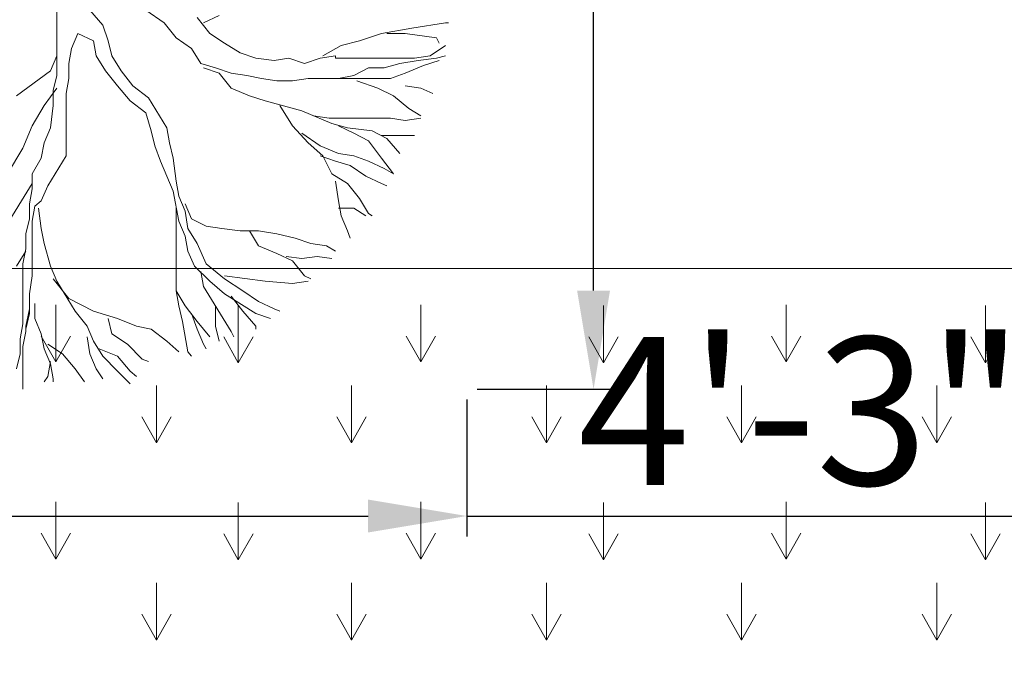
# Model space of a CAD drawing. Units: millimetres. Extents: x 595116 to 630915, y 909473 to 920225.
# Tile 50 of 134: x 629559 to 629619, y 919242 to 919281. Entities that reach past the tile are written whole.
import ezdxf

# ---------------------------------------------------------------- set-up
doc = ezdxf.new("R2010")
doc.units = ezdxf.units.MM
doc.layers.add('Dimension', color=3, linetype='Continuous', lineweight=18)
doc.layers.add('L-PLNT', color=85, linetype='Continuous', lineweight=13)
doc.styles.get("Standard").update_dxf_attribs({"font": 'arial.ttf'})
doc.dimstyles.new('ISO-25', dxfattribs={"dimtxt": 9, "dimasz": 6, "dimexe": 1.25, "dimexo": 0.625, "dimtad": 1, "dimlunit": 4, "dimtxsty": 'Standard', "dimcen": 2.5, "dimadec": 0, "dimazin": 0, "dimtfac": 1, "dimtmove": 0, "dimatfit": 3, "dimfxl": 1, "dimarcsym": 0})

# ---------------------------------------------------------------- blocks, each defined once
blk = doc.blocks.new('A$C143125F4')
for p, q in [((2.5383, 1.8726), (2.5383, 2.3206)), ((2.7353, 2.2623), (2.8119, 2.1727)), ((3.1784, 2.1862), (3.069, 2.2623)), ((3.2495, 2.0966), (3.1784, 2.1862)), ((3.4519, 2.1235), (3.3753, 2.2175)), ((3.4136, 2.1862), (3.5066, 2.231)), ((4.6554, 2.1548), (4.8578, 2.1862)), ((4.8578, 2.1862), (4.8742, 2.1862)), ((2.6641, 2.1235), (2.6259, 2.0339)), ((2.7571, 2.0787), (2.6641, 2.1235)), ((2.8119, 2.1727), (2.8447, 2.0787)), ((3.5394, 2.0652), (3.4519, 2.1235)), ((4.3436, 2.0787), (4.4749, 2.1235)), ((4.4749, 2.1235), (4.6554, 2.1548)), ((4.5077, 2.1235), (4.6171, 2.1235)), ((4.6171, 2.1235), (4.8031, 2.0966)), ((2.7736, 1.9891), (2.7571, 2.0787)), ((2.8447, 2.0787), (2.8666, 1.9891)), ((3.3425, 2.0339), (3.2495, 2.0966)), ((3.6324, 2.007), (3.5394, 2.0652)), ((4.2342, 2.0518), (4.3436, 2.0787)), ((4.8031, 2.0966), (4.8195, 2.0652)), ((2.6259, 2.0339), (2.6094, 1.9443)), ((3.3972, 1.9443), (3.3425, 2.0339)), ((3.7254, 1.9756), (3.6324, 2.007)), ((4.1248, 1.9891), (4.2342, 2.0518)), ((4.8578, 2.0518), (4.7648, 1.9891)), ((2.5383, 1.9891), (2.5, 1.8995)), ((2.6094, 1.9443), (2.6094, 1.8547)), ((2.8283, 1.8995), (2.7736, 1.9891)), ((2.8666, 1.9891), (2.9213, 1.8995)), ((3.4847, 1.9174), (3.3972, 1.9443)), ((3.8348, 1.9622), (3.7254, 1.9756)), ((3.9224, 1.9756), (3.8348, 1.9622)), ((4.0154, 1.9443), (3.9224, 1.9756)), ((4.1084, 1.9756), (4.0154, 1.9443)), ((4.2014, 1.9891), (4.1084, 1.9756)), ((4.2014, 1.9756), (4.2014, 1.9891)), ((4.6718, 1.9756), (4.2014, 1.9756)), ((4.4913, 1.9174), (4.5843, 1.9443)), ((4.5843, 1.9443), (4.6937, 1.9622)), ((4.7648, 1.9891), (4.6718, 1.9756)), ((4.6937, 1.9622), (4.8031, 1.9756)), ((4.8195, 1.9622), (4.7265, 1.9308)), ((4.8031, 1.9756), (4.8578, 1.9891)), ((2.5, 1.8995), (2.2976, 1.7516)), ((2.8994, 1.8099), (2.8283, 1.8995)), ((2.9213, 1.8995), (2.9924, 1.8099)), ((3.4136, 1.9174), (3.5066, 1.886)), ((3.5777, 1.886), (3.4847, 1.9174)), ((3.5066, 1.886), (3.5777, 1.7964)), ((3.6707, 1.8726), (3.5777, 1.886)), ((4.3108, 1.8726), (4.3983, 1.9174)), ((4.3983, 1.9174), (4.4913, 1.9174)), ((4.6171, 1.886), (4.5296, 1.8547)), ((4.7265, 1.9308), (4.6171, 1.886)), ((2.5164, 1.783), (2.5383, 1.8726)), ((2.6094, 1.8547), (2.593, 1.7651)), ((3.7583, 1.8547), (3.6707, 1.8726)), ((3.8512, 1.8412), (3.7583, 1.8547)), ((3.9442, 1.8412), (3.8512, 1.8412)), ((4.0372, 1.8547), (3.9442, 1.8412)), ((4.1248, 1.8547), (4.0372, 1.8547)), ((4.5296, 1.8547), (4.1248, 1.8547)), ((4.2178, 1.8547), (4.3108, 1.8726)), ((4.3272, 1.8412), (4.453, 1.7964)), ((2.5383, 1.7964), (2.4617, 1.6934)), ((2.5164, 1.6934), (2.5164, 1.783)), ((2.593, 1.7651), (2.593, 1.3932)), ((2.976, 1.7203), (2.8994, 1.8099)), ((2.9924, 1.8099), (3.0854, 1.7382)), ((3.5777, 1.7964), (3.6871, 1.7516)), ((4.453, 1.7964), (4.546, 1.7516)), ((4.6171, 1.8099), (4.7101, 1.7964)), ((4.7101, 1.7964), (4.7812, 1.7651)), ((3.069, 1.6486), (2.976, 1.7203)), ((3.0854, 1.7382), (3.1948, 1.559)), ((3.6871, 1.7516), (3.7801, 1.7203)), ((3.7801, 1.7203), (3.999, 1.662)), ((4.546, 1.7516), (4.639, 1.6755)), ((2.4617, 1.6934), (2.3906, 1.5724)), ((2.5, 1.559), (2.5164, 1.6934)), ((3.1018, 1.5411), (3.069, 1.6486)), ((3.8677, 1.6934), (3.9442, 1.5724)), ((3.999, 1.662), (4.1795, 1.5859)), ((4.639, 1.6755), (4.7101, 1.6307)), ((4.0701, 1.6307), (4.1631, 1.6172)), ((4.1631, 1.6172), (4.5296, 1.6172)), ((4.5296, 1.6172), (4.6171, 1.6038)), ((4.6171, 1.6038), (4.7101, 1.6172)), ((2.3906, 1.5724), (2.3359, 1.438)), ((2.4617, 1.4694), (2.5, 1.559)), ((3.1237, 1.4515), (3.1018, 1.5411)), ((3.1948, 1.559), (3.2112, 1.4694)), ((3.9442, 1.5724), (4.0372, 1.4694)), ((3.999, 1.5276), (4.1084, 1.4515)), ((4.1795, 1.5859), (4.2725, 1.559)), ((4.2178, 1.5724), (4.3108, 1.5276)), ((4.2725, 1.559), (4.4202, 1.5411)), ((4.3108, 1.5276), (4.3983, 1.4828)), ((4.4202, 1.5411), (4.5077, 1.4963)), ((2.4453, 1.3798), (2.4617, 1.4694)), ((3.2112, 1.4694), (3.2331, 1.3798)), ((4.0372, 1.4694), (4.1248, 1.3932)), ((4.3983, 1.4828), (4.4749, 1.3798)), ((4.4749, 1.5142), (4.6718, 1.5142)), ((4.5077, 1.4963), (4.5843, 1.4067)), ((2.3359, 1.438), (2.2429, 1.2857)), ((3.1565, 1.3619), (3.1237, 1.4515)), ((4.1084, 1.4515), (4.2178, 1.4067)), ((2.3906, 1.2857), (2.4453, 1.3798)), ((2.593, 1.3932), (2.4836, 1.214)), ((3.2331, 1.1827), (3.1565, 1.3619)), ((3.2331, 1.3798), (3.2495, 1.2409)), ((4.1084, 1.3932), (4.2014, 1.3619)), ((4.1248, 1.3932), (4.1795, 1.2857)), ((4.2014, 1.3619), (4.2889, 1.335)), ((4.2178, 1.4067), (4.3108, 1.3932)), ((4.3108, 1.3932), (4.3983, 1.3619)), ((4.3983, 1.3619), (4.4913, 1.3171)), ((4.4749, 1.3798), (4.546, 1.2857)), ((4.2889, 1.335), (4.3819, 1.2723)), ((4.4913, 1.3171), (4.546, 1.2857)), ((2.3906, 1.1961), (2.3906, 1.2857)), ((3.2495, 1.2409), (3.2659, 1.1513)), ((4.1795, 1.2857), (4.2725, 1.2275)), ((4.2014, 1.2409), (4.2178, 1.1244)), ((4.3819, 1.2723), (4.4749, 1.2275)), ((2.3906, 1.2275), (2.2265, 0.9587)), ((2.3742, 1.1065), (2.3906, 1.1961)), ((2.4836, 1.214), (2.4453, 1.1244)), ((3.2659, 1.0035), (3.2331, 1.1827)), ((4.2725, 1.2275), (4.3436, 1.1379)), ((4.4749, 1.2275), (4.5077, 1.214)), ((2.4453, 1.1244), (2.407, 1.0931)), ((3.2659, 1.1513), (3.3042, 1.0617)), ((4.2178, 1.1244), (4.2342, 1.0348)), ((4.3436, 1.1379), (4.3983, 1.0483)), ((2.3742, 1.0169), (2.3742, 1.1065)), ((2.407, 1.0931), (2.3906, 1.0035)), ((2.4289, 1.0796), (2.4453, 0.9587)), ((3.2495, 1.0796), (3.2495, 0.5869)), ((3.3042, 1.1065), (3.3425, 1.0169)), ((3.3042, 1.0617), (3.3206, 0.9587)), ((4.2178, 1.0796), (4.3108, 1.0796)), ((4.3108, 1.0796), (4.3819, 1.0348)), ((2.3523, 0.9273), (2.3742, 1.0169)), ((2.3906, 1.0035), (2.3906, 0.6765)), ((3.3042, 0.9139), (3.2659, 1.0035)), ((3.3425, 1.0169), (3.43, 0.9721)), ((4.2342, 1.0348), (4.2725, 0.9452)), ((4.3983, 1.0483), (4.4202, 1.0348)), ((2.4453, 0.9587), (2.4617, 0.8691)), ((3.3206, 0.9587), (3.3753, 0.8691)), ((3.43, 0.9721), (3.523, 0.9587)), ((3.523, 0.9587), (3.6324, 0.9452)), ((3.6324, 0.9452), (3.7418, 0.9452)), ((3.6871, 0.9452), (3.7418, 0.8557)), ((3.7418, 0.9452), (3.8512, 0.9273)), ((4.2725, 0.9452), (4.2889, 0.9005)), ((2.3523, 0.8377), (2.3523, 0.9273)), ((3.3206, 0.8243), (3.3042, 0.9139)), ((3.8512, 0.9273), (3.9607, 0.9005)), ((3.9607, 0.9005), (4.0537, 0.8691)), ((2.3523, 0.8243), (2.2976, 0.7347)), ((2.3359, 0.7481), (2.3523, 0.8377)), ((2.4617, 0.8691), (2.5, 0.7347)), ((3.3589, 0.7347), (3.3206, 0.8243)), ((3.3753, 0.8691), (3.43, 0.7481)), ((3.7418, 0.8557), (3.8512, 0.8109)), ((4.0537, 0.8691), (4.1467, 0.8557)), ((4.1467, 0.8557), (4.2014, 0.8243)), ((3.8512, 0.8109), (3.9442, 0.7661)), ((3.906, 0.7929), (3.999, 0.7795)), ((3.9442, 0.7661), (4.0154, 0.6765)), ((3.999, 0.7795), (4.092, 0.7929)), ((4.092, 0.7929), (4.1795, 0.7795)), ((2.3359, 0.3897), (2.3359, 0.7481)), ((2.5, 0.7347), (2.5383, 0.6451)), ((3.4519, 0.6451), (3.3589, 0.7347)), ((3.43, 0.7481), (3.5394, 0.6585)), ((2.3906, 0.6765), (2.3742, 0.5689)), ((2.5164, 0.6585), (2.6094, 0.5421)), ((3.3972, 0.7033), (3.4136, 0.6137)), ((3.5394, 0.6765), (3.7801, 0.6451)), ((3.5394, 0.6585), (3.6488, 0.5869)), ((4.0154, 0.6765), (4.0537, 0.6585)), ((2.5383, 0.6451), (2.6477, 0.4659)), ((3.4136, 0.6137), (3.5777, 0.3449)), ((3.5394, 0.5689), (3.4519, 0.6451)), ((3.7801, 0.6451), (3.9442, 0.6317)), ((3.9442, 0.6317), (4.0372, 0.6451)), ((2.3742, 0.5689), (2.3742, 0.4525)), ((2.6094, 0.5421), (2.7571, 0.4659)), ((3.2495, 0.5869), (3.3042, 0.4973)), ((3.2495, 0.5869), (3.2659, 0.4973)), ((3.7254, 0.4525), (3.5394, 0.5689)), ((3.5777, 0.5555), (3.6488, 0.4659)), ((3.6488, 0.5869), (3.7418, 0.5241)), ((2.3523, 0.3584), (2.3742, 0.4793)), ((2.3742, 0.4793), (2.3523, 0.3763)), ((2.407, 0.5107), (2.407, 0.4211)), ((3.2659, 0.4973), (3.2878, 0.4032)), ((3.3042, 0.4973), (3.3753, 0.4032)), ((3.4847, 0.4973), (3.4847, 0.3763)), ((3.7418, 0.5241), (3.8348, 0.4793)), ((3.8348, 0.4793), (3.8677, 0.4659)), ((2.3742, 0.4525), (2.3523, 0.3584)), ((2.407, 0.4211), (2.4453, 0.3315)), ((2.6477, 0.4659), (2.7189, 0.3763)), ((2.7571, 0.4659), (2.8994, 0.4211)), ((2.8447, 0.4211), (2.8666, 0.3315)), ((2.8994, 0.4211), (3.0143, 0.3763)), ((3.3425, 0.4525), (3.3753, 0.3584)), ((3.6488, 0.4659), (3.7254, 0.3763)), ((3.813, 0.4211), (3.7254, 0.4525)), ((2.3195, 0.3002), (2.3359, 0.3897)), ((2.3523, 0.3763), (2.3523, 0.3449)), ((2.7189, 0.3763), (2.7571, 0.2867)), ((3.0143, 0.3763), (3.1018, 0.3584)), ((3.1018, 0.3584), (3.1948, 0.2867)), ((3.2878, 0.4032), (3.3206, 0.224)), ((3.3753, 0.4032), (3.4519, 0.3136)), ((3.3753, 0.3584), (3.4136, 0.2688)), ((3.4847, 0.3763), (3.5066, 0.2867)), ((3.7254, 0.3763), (3.7254, 0.3584)), ((2.3195, 0.2106), (2.3195, 0.3002)), ((2.3523, 0.3449), (2.3359, 0.2554)), ((2.4453, 0.3315), (2.4617, 0.2419)), ((2.7189, 0.3136), (2.7353, 0.2106)), ((2.8666, 0.3315), (2.9596, 0.2688)), ((3.5777, 0.3449), (3.5941, 0.3136)), ((2.3359, 0.2554), (2.3359, 0)), ((2.4617, 0.2419), (2.5, 0.1523)), ((2.4836, 0.2688), (2.5711, 0.2106)), ((2.7571, 0.2867), (2.8119, 0.1971)), ((2.79, 0.2419), (2.8994, 0.1971)), ((2.9596, 0.2688), (3.0471, 0.1792)), ((3.1948, 0.2867), (3.2659, 0.224)), ((3.4136, 0.2688), (3.43, 0.2419)), ((2.2976, 0.121), (2.3195, 0.2106)), ((2.5711, 0.2106), (2.6477, 0.121)), ((2.7353, 0.2106), (2.7736, 0.121)), ((2.8119, 0.1971), (2.8994, 0.1075)), ((2.8994, 0.1971), (2.976, 0.1075)), ((3.0471, 0.1792), (3.0854, 0.1658)), ((3.3206, 0.224), (3.3425, 0.1971)), ((2.5, 0.1658), (2.4836, 0.0762)), ((2.5, 0.1523), (2.5164, 0.0627)), ((2.6477, 0.121), (2.7024, 0.0448)), ((2.7736, 0.121), (2.8119, 0.0627)), ((2.4836, 0.0762), (2.4617, 0.0448)), ((2.5164, 0.0627), (2.5164, 0.0448)), ((2.8994, 0.1075), (2.976, 0.0314)), ((2.976, 0.1075), (3.0143, 0.0762))]:
    blk.add_line(p, q)
blk = doc.blocks.new('LAWN-GRASS-TUFT')
blk.add_line((0.892, 3.485), (0.892, 0))
blk.add_lwpolyline([(0, 1.577), (0.892, 0), (1.785, 1.577)])
blk = doc.blocks.new('*D210')
at = {"layer": 'Defpoints', "color": 0, "transparency": 16777216}
for p in [(629586.227, 919310.123), (629593.946, 919310.123), (629586.227, 919258.662)]:
    blk.add_point(p, dxfattribs=at)
at = {"layer": 'Dimension', "color": 0, "lineweight": -2, "transparency": 16777216}
for p, q in [((629593.946, 919310.123), (629593.946, 919449.69)), ((629586.852, 919310.123), (629595.196, 919310.123)), ((629593.946, 919264.662), (629593.946, 919304.123)), ((629586.852, 919258.662), (629595.196, 919258.662))]:
    blk.add_line(p, q, dxfattribs=at)
at = {"layer": 'Dimension', "color": 0, "transparency": 16777216}
for points in [[(629592.946, 919304.123), (629594.946, 919304.123), (629593.946, 919310.123)], [(629592.946, 919264.662), (629594.946, 919264.662), (629593.946, 919258.662)]]:
    blk.add_solid(points, dxfattribs=at)
at = {"layer": 'Dimension', "color": 0, "transparency": 16777216, "insert": (629588.662, 919382.907), "char_height": 9, "attachment_point": 5, "rotation": 90}
blk.add_mtext('CANOPY 4\'-3 1/2" TYP.', dxfattribs=at)
blk = doc.blocks.new('*D211')
at = {"layer": 'Defpoints', "color": 0, "transparency": 16777216}
for p in [(629535.386, 919258.662), (629586.227, 919258.662), (629586.227, 919250.943)]:
    blk.add_point(p, dxfattribs=at)
at = {"layer": 'Dimension', "color": 0, "lineweight": -2, "transparency": 16777216}
for p, q in [((629535.386, 919258.037), (629535.386, 919249.693)), ((629586.227, 919258.037), (629586.227, 919249.693)), ((629541.386, 919250.943), (629580.227, 919250.943)), ((629586.227, 919250.943), (629648.699, 919250.943))]:
    blk.add_line(p, q, dxfattribs=at)
at = {"layer": 'Dimension', "color": 0, "transparency": 16777216}
for points in [[(629541.386, 919251.943), (629541.386, 919249.943), (629535.386, 919250.943)], [(629580.227, 919251.943), (629580.227, 919249.943), (629586.227, 919250.943)]]:
    blk.add_solid(points, dxfattribs=at)
at = {"layer": 'Dimension', "color": 0, "transparency": 16777216, "insert": (629620.463, 919256.167), "char_height": 9, "attachment_point": 5}
blk.add_mtext('4\'-3" TYP.', dxfattribs=at)
blk = doc.blocks.new('*D216')
at = {"layer": 'Defpoints', "color": 0, "transparency": 16777216}
for p in [(629505.041, 919411.828), (629743.541, 919411.928), (629743.541, 918832.378)]:
    blk.add_point(p, dxfattribs=at)
at = {"layer": 'Dimension', "color": 0, "lineweight": -2, "transparency": 16777216}
for p, q in [((629505.041, 919411.203), (629505.041, 918831.128)), ((629743.541, 919411.303), (629743.541, 918831.128)), ((629511.041, 918832.378), (629737.541, 918832.378))]:
    blk.add_line(p, q, dxfattribs=at)
at = {"layer": 'Dimension', "color": 0, "transparency": 16777216}
for points in [[(629511.041, 918833.378), (629511.041, 918831.378), (629505.041, 918832.378)], [(629737.541, 918833.378), (629737.541, 918831.378), (629743.541, 918832.378)]]:
    blk.add_solid(points, dxfattribs=at)
at = {"layer": 'Dimension', "color": 0, "transparency": 16777216, "insert": (629624.291, 918837.656), "char_height": 9, "attachment_point": 5}
blk.add_mtext('19\'-10 1/2"', dxfattribs=at)

msp = doc.modelspace()

# ---------------------------------------------------------------- linework, layer by layer
at = {"layer": 'L-PLNT'}
msp.add_line((629800.951, 919266.009), (629535.274, 919266.009), dxfattribs=at)

# ---------------------------------------------------------------- block references
at = {"layer": 'L-PLNT', "xscale": 10.20167662382051, "yscale": 10.20167662382051, "zscale": 10.20167662382051}
msp.add_blockref('A$C143125F4', (629535.386, 919258.662), dxfattribs=at)
at = {"layer": 'L-PLNT'}
for p in [(629560.321, 919260.324), (629571.434, 919260.275), (629582.548, 919260.324), (629593.662, 919260.275), (629604.776, 919260.324), (629616.912, 919260.275), (629566.446, 919255.397), (629578.319, 919255.397), (629590.192, 919255.397), (629602.065, 919255.397), (629613.938, 919255.397), (629560.321, 919248.322), (629571.434, 919248.272), (629582.548, 919248.322), (629593.662, 919248.272), (629604.776, 919248.322), (629616.912, 919248.272), (629566.446, 919243.395), (629578.319, 919243.395), (629590.192, 919243.395), (629602.065, 919243.395), (629613.938, 919243.395)]:
    msp.add_blockref('LAWN-GRASS-TUFT', p, dxfattribs=at)

# ---------------------------------------------------------------- dimensions: what is measured, and where the dimension line sits
at = {"layer": 'Dimension'}
dim = msp.add_linear_dim(base=(629593.946, 919310.123), p1=(629586.227, 919258.662), p2=(629586.227, 919310.123), angle=90, text='CANOPY <> TYP.', dimstyle='ISO-25', override={"dimdec": 1, "dimlfac": 1, "dimrnd": 0, "dimzin": 1, "dimdsep": 46, "dimlunit": 4, "dimfrac": 2}, dxfattribs=at)
dim.commit()
dim.dimension.update_dxf_attribs({"geometry": '*D210', "text_midpoint": (629588.662, 919382.907)})
dim = msp.add_linear_dim(base=(629743.541, 918832.378), p1=(629505.041, 919411.828), p2=(629743.541, 919411.928), dimstyle='ISO-25', override={"dimdec": 1, "dimlfac": 1, "dimrnd": 0, "dimzin": 1, "dimdsep": 46, "dimlunit": 4, "dimfrac": 2}, dxfattribs=at)
dim.commit()
dim.dimension.update_dxf_attribs({"geometry": '*D216', "text_midpoint": (629624.291, 918837.656)})
dim = msp.add_linear_dim(base=(629586.227, 919250.943), p1=(629535.386, 919258.662), p2=(629586.227, 919258.662), text='<> TYP.', dimstyle='ISO-25', override={"dimdec": 1, "dimlfac": 1, "dimrnd": 0, "dimzin": 1, "dimdsep": 46, "dimlunit": 4, "dimfrac": 2}, dxfattribs=at)
dim.commit()
dim.dimension.update_dxf_attribs({"geometry": '*D211', "text_midpoint": (629620.463, 919256.167)})

doc.saveas('drawing.dxf')
